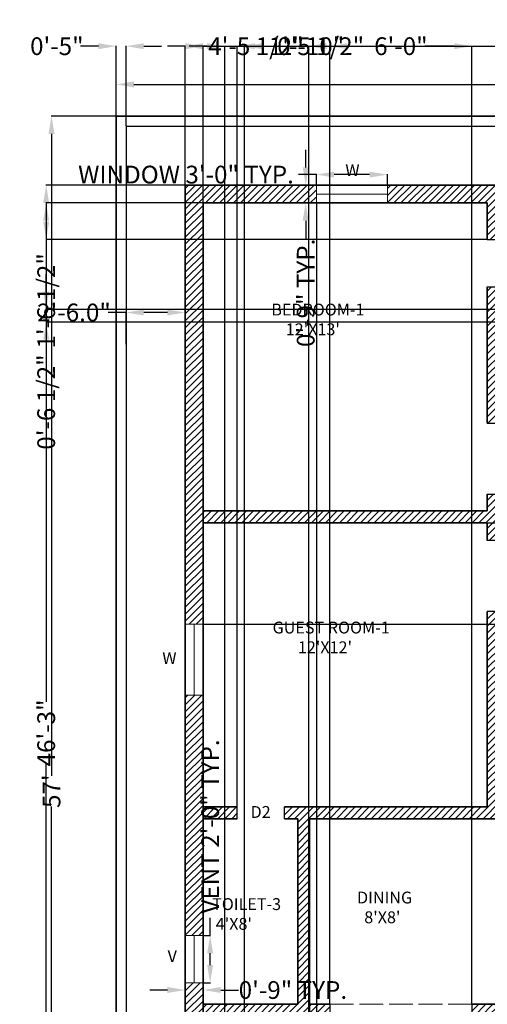
# Model space of a CAD drawing. Units: inches. Extents: x 287 to 864, y 208 to 990.
# Tile 2 of 3: x 287 to 524, y 491 to 990. Entities that reach past the tile are written whole.
import ezdxf

# ---------------------------------------------------------------- set-up
doc = ezdxf.new("R2010")
doc.units = ezdxf.units.IN
doc.header["$MEASUREMENT"] = 0
doc.linetypes.add('ACAD_ISO02W100', pattern=[15, 12, -3])
for name, color, linetype, lineweight in [('A-ANNO-DIMS', 2, 'Continuous', 18), ('A-ANNO-TEXT', 7, 'Continuous', 18), ('A-AREA-IDEN', 7, 'Continuous', 18), ('A-DOOR', 3, 'Continuous', 25), ('A-GLAZ', 4, 'Continuous', 18), ('A-SITE-WALL', 7, 'Continuous', 30), ('A-WALL', 7, 'Continuous', 35), ('A-WALL-OVHD', 7, 'ACAD_ISO02W100', 18), ('C-PROP', 7, 'Continuous', 35)]:
    doc.layers.add(name, color=color, linetype=linetype, lineweight=lineweight)
doc.layers.add('A-WALL-PATT', color=240, linetype='Continuous', lineweight=13, true_color=0xed1f24)
doc.styles.get("Standard").update_dxf_attribs({"font": 'arial.ttf'})
doc.dimstyles.get("Standard").update_dxf_attribs({"dimtxt": 9, "dimasz": 9, "dimexe": 0.18, "dimexo": 0.0625, "dimgap": 0.09, "dimtad": 0, "dimdec": 1, "dimzin": 0, "dimdsep": 46, "dimlunit": 3, "dimtxsty": 'Standard', "dimcen": 0.09, "dimadec": 0, "dimazin": 0, "dimtfac": 1, "dimtdec": 1, "dimtofl": 0, "dimtmove": 0, "dimatfit": 3, "dimfxl": 1, "dimtolj": 1, "dimtzin": 0, "dimarcsym": 0})

# ---------------------------------------------------------------- blocks, each defined once
blk = doc.blocks.new('*D1')
at = {"layer": 'A-ANNO-DIMS', "color": 0, "lineweight": -2, "transparency": 16777216}
for p, q in [((335.59, 941.12), (335.59, 957.32)), ((344.59, 957.14), (567.68, 957.14)), ((806.59, 957.14), (583.5, 957.14)), ((815.59, 941.12), (815.59, 957.32))]:
    blk.add_line(p, q, dxfattribs=at)
at = {"layer": 'A-ANNO-DIMS', "color": 0, "transparency": 16777216}
for points in [[(344.59, 958.64), (344.59, 955.64), (335.59, 957.14)], [(806.59, 958.64), (806.59, 955.64), (815.59, 957.14)]]:
    blk.add_solid(points, dxfattribs=at)
at = {"layer": 'Defpoints', "color": 0, "transparency": 16777216}
for p in [(815.59, 957.14), (335.59, 941.05), (815.59, 941.05)]:
    blk.add_point(p, dxfattribs=at)
at = {"layer": 'A-ANNO-DIMS', "color": 0, "transparency": 16777216, "insert": (575.59, 957.14), "char_height": 9, "attachment_point": 5}
blk.add_mtext("\\A1;40'", dxfattribs=at)
blk = doc.blocks.new('*D2')
at = {"layer": 'A-ANNO-DIMS', "color": 0, "lineweight": -2, "transparency": 16777216}
for p, q in [((335.53, 941.05), (302.65, 941.05)), ((302.83, 932.05), (302.83, 606.78)), ((302.83, 266.05), (302.83, 591.33)), ((335.53, 257.05), (302.65, 257.05))]:
    blk.add_line(p, q, dxfattribs=at)
at = {"layer": 'A-ANNO-DIMS', "color": 0, "transparency": 16777216}
for points in [[(301.33, 932.05), (304.33, 932.05), (302.83, 941.05)], [(301.33, 266.05), (304.33, 266.05), (302.83, 257.05)]]:
    blk.add_solid(points, dxfattribs=at)
at = {"layer": 'Defpoints', "color": 0, "transparency": 16777216}
for p in [(335.59, 941.05), (302.83, 257.05), (335.59, 257.05)]:
    blk.add_point(p, dxfattribs=at)
at = {"layer": 'A-ANNO-DIMS', "color": 0, "transparency": 16777216, "insert": (302.83, 599.05), "char_height": 9, "attachment_point": 5, "rotation": 90}
blk.add_mtext("\\A1;57'", dxfattribs=at)
blk = doc.blocks.new('*D3')
at = {"layer": 'A-ANNO-DIMS', "color": 0, "lineweight": -2, "transparency": 16777216}
for p, q in [((340.59, 841.58), (331.59, 841.58)), ((340.59, 825.53), (340.59, 841.76)), ((361.59, 841.58), (349.59, 841.58)), ((370.59, 825.53), (370.59, 841.76))]:
    blk.add_line(p, q, dxfattribs=at)
at = {"layer": 'A-ANNO-DIMS', "color": 0, "transparency": 16777216}
for points in [[(349.59, 843.08), (349.59, 840.08), (340.59, 841.58)], [(361.59, 843.08), (361.59, 840.08), (370.59, 841.58)]]:
    blk.add_solid(points, dxfattribs=at)
at = {"layer": 'Defpoints', "color": 0, "transparency": 16777216}
for p in [(340.59, 841.58), (340.59, 825.47), (370.59, 825.47)]:
    blk.add_point(p, dxfattribs=at)
at = {"layer": 'A-ANNO-DIMS', "color": 0, "transparency": 16777216, "insert": (314.22, 841.58), "char_height": 9, "attachment_point": 5}
blk.add_mtext('\\A1;2\'-6.0"', dxfattribs=at)
blk = doc.blocks.new('WIN-36IN')
for p, q in [((0, 9), (0, 0)), ((36, 9), (36, 0)), ((0, 4.5), (36, 4.5))]:
    blk.add_line(p, q)
blk = doc.blocks.new('VENT-24IN')
for p, q in [((0, 24), (9, 24)), ((4.5, 0), (4.5, 24)), ((0, 0), (9, 0))]:
    blk.add_line(p, q)
blk = doc.blocks.new('DOOR-OPENING-36IN')
for p, q in [((0, 36), (6, 36)), ((0, 0), (6, 0))]:
    blk.add_line(p, q)
blk = doc.blocks.new('DOOR-OPENING-24IN')
for p, q in [((0, 24), (6, 24)), ((0, 0), (6, 0))]:
    blk.add_line(p, q)
blk = doc.blocks.new('*D13')
at = {"layer": 'A-ANNO-DIMS', "color": 0, "lineweight": -2, "transparency": 16777216}
for p, q in [((436.99, 911.45), (427.99, 911.45)), ((436.99, 906.12), (436.99, 911.63)), ((463.99, 911.45), (445.99, 911.45)), ((472.99, 906.12), (472.99, 911.63))]:
    blk.add_line(p, q, dxfattribs=at)
at = {"layer": 'A-ANNO-DIMS', "color": 0, "transparency": 16777216}
for points in [[(445.99, 912.95), (445.99, 909.95), (436.99, 911.45)], [(463.99, 912.95), (463.99, 909.95), (472.99, 911.45)]]:
    blk.add_solid(points, dxfattribs=at)
at = {"layer": 'Defpoints', "color": 0, "transparency": 16777216}
for p in [(436.99, 911.45), (436.99, 906.05), (472.99, 906.05)]:
    blk.add_point(p, dxfattribs=at)
at = {"layer": 'A-ANNO-DIMS', "color": 0, "transparency": 16777216, "insert": (370.96, 911.45), "char_height": 9, "attachment_point": 5}
blk.add_mtext('\\A1;WINDOW 3\'-0" TYP.', dxfattribs=at)
blk = doc.blocks.new('*D14')
at = {"layer": 'A-ANNO-DIMS', "color": 0, "lineweight": -2, "transparency": 16777216}
for p, q in [((431.59, 915.05), (431.59, 924.05)), ((436.93, 906.05), (431.41, 906.05)), ((436.93, 897.05), (431.41, 897.05)), ((431.59, 888.05), (431.59, 879.05))]:
    blk.add_line(p, q, dxfattribs=at)
at = {"layer": 'A-ANNO-DIMS', "color": 0, "transparency": 16777216}
for points in [[(430.09, 915.05), (433.09, 915.05), (431.59, 906.05)], [(430.09, 888.05), (433.09, 888.05), (431.59, 897.05)]]:
    blk.add_solid(points, dxfattribs=at)
at = {"layer": 'Defpoints', "color": 0, "transparency": 16777216}
for p in [(436.99, 906.05), (431.59, 897.05), (436.99, 897.05)]:
    blk.add_point(p, dxfattribs=at)
at = {"layer": 'A-ANNO-DIMS', "color": 0, "transparency": 16777216, "insert": (431.59, 851.53), "char_height": 9, "attachment_point": 5, "rotation": 90}
blk.add_mtext('\\A1;0\'-9" TYP.', dxfattribs=at)
blk = doc.blocks.new('*D19')
at = {"layer": 'A-ANNO-DIMS', "color": 0, "lineweight": -2, "transparency": 16777216}
for p, q in [((383.19, 525.9), (383.19, 534.9)), ((379.65, 525.9), (383.37, 525.9)), ((383.19, 510.9), (383.19, 516.9)), ((379.65, 501.9), (383.37, 501.9))]:
    blk.add_line(p, q, dxfattribs=at)
at = {"layer": 'A-ANNO-DIMS', "color": 0, "transparency": 16777216}
for points in [[(381.69, 516.9), (384.69, 516.9), (383.19, 525.9)], [(381.69, 510.9), (384.69, 510.9), (383.19, 501.9)]]:
    blk.add_solid(points, dxfattribs=at)
at = {"layer": 'Defpoints', "color": 0, "transparency": 16777216}
for p in [(379.59, 525.9), (383.19, 525.9), (379.59, 501.9)]:
    blk.add_point(p, dxfattribs=at)
at = {"layer": 'A-ANNO-DIMS', "color": 0, "transparency": 16777216, "insert": (383.19, 581.17), "char_height": 9, "attachment_point": 5, "rotation": 90}
blk.add_mtext('\\A1;VENT 2\'-0" TYP.', dxfattribs=at)
blk = doc.blocks.new('*D20')
at = {"layer": 'A-ANNO-DIMS', "color": 0, "lineweight": -2, "transparency": 16777216}
for p, q in [((370.59, 501.84), (370.59, 498.12)), ((379.59, 501.84), (379.59, 498.12)), ((361.59, 498.3), (352.59, 498.3)), ((388.59, 498.3), (397.59, 498.3))]:
    blk.add_line(p, q, dxfattribs=at)
at = {"layer": 'A-ANNO-DIMS', "color": 0, "transparency": 16777216}
for points in [[(361.59, 499.8), (361.59, 496.8), (370.59, 498.3)], [(388.59, 499.8), (388.59, 496.8), (379.59, 498.3)]]:
    blk.add_solid(points, dxfattribs=at)
at = {"layer": 'Defpoints', "color": 0, "transparency": 16777216}
for p in [(370.59, 501.9), (379.59, 501.9), (379.59, 498.3)]:
    blk.add_point(p, dxfattribs=at)
at = {"layer": 'A-ANNO-DIMS', "color": 0, "transparency": 16777216, "insert": (425.11, 498.3), "char_height": 9, "attachment_point": 5}
blk.add_mtext('\\A1;0\'-9" TYP.', dxfattribs=at)
blk = doc.blocks.new('*D23')
at = {"layer": 'A-ANNO-DIMS', "color": 0, "lineweight": -2, "transparency": 16777216}
for p, q in [((370.59, 906.12), (370.59, 976.68)), ((379.59, 976.5), (556.04, 976.5)), ((763.59, 976.5), (587.14, 976.5)), ((772.59, 906.12), (772.59, 976.68))]:
    blk.add_line(p, q, dxfattribs=at)
at = {"layer": 'A-ANNO-DIMS', "color": 0, "transparency": 16777216}
for points in [[(379.59, 978), (379.59, 975), (370.59, 976.5)], [(763.59, 978), (763.59, 975), (772.59, 976.5)]]:
    blk.add_solid(points, dxfattribs=at)
at = {"layer": 'Defpoints', "color": 0, "transparency": 16777216}
for p in [(772.59, 976.5), (370.59, 906.05), (772.59, 906.05)]:
    blk.add_point(p, dxfattribs=at)
at = {"layer": 'A-ANNO-DIMS', "color": 0, "transparency": 16777216, "insert": (571.59, 976.5), "char_height": 9, "attachment_point": 5}
blk.add_mtext('\\A1;33\'-6"', dxfattribs=at)
blk = doc.blocks.new('*D24')
at = {"layer": 'A-ANNO-DIMS', "color": 0, "lineweight": -2, "transparency": 16777216}
for p, q in [((370.53, 906.05), (299.96, 906.05)), ((300.14, 897.05), (300.14, 644.28)), ((300.14, 360.05), (300.14, 612.83)), ((370.53, 351.05), (299.96, 351.05))]:
    blk.add_line(p, q, dxfattribs=at)
at = {"layer": 'A-ANNO-DIMS', "color": 0, "transparency": 16777216}
for points in [[(298.64, 897.05), (301.64, 897.05), (300.14, 906.05)], [(298.64, 360.05), (301.64, 360.05), (300.14, 351.05)]]:
    blk.add_solid(points, dxfattribs=at)
at = {"layer": 'Defpoints', "color": 0, "transparency": 16777216}
for p in [(300.14, 906.05), (370.59, 906.05), (370.59, 351.05)]:
    blk.add_point(p, dxfattribs=at)
at = {"layer": 'A-ANNO-DIMS', "color": 0, "transparency": 16777216, "insert": (300.14, 628.55), "char_height": 9, "attachment_point": 5, "rotation": 90}
blk.add_mtext('\\A1;46\'-3"', dxfattribs=at)
blk = doc.blocks.new('*D28')
at = {"layer": 'A-ANNO-DIMS', "color": 0, "lineweight": -2, "transparency": 16777216}
for p, q in [((381.59, 976.5), (372.59, 976.5)), ((390.59, 351.12), (390.59, 976.68)), ((400.59, 351.12), (400.59, 976.68)), ((409.59, 976.5), (418.59, 976.5))]:
    blk.add_line(p, q, dxfattribs=at)
at = {"layer": 'A-ANNO-DIMS', "color": 0, "transparency": 16777216}
for points in [[(381.59, 978), (381.59, 975), (390.59, 976.5)], [(409.59, 978), (409.59, 975), (400.59, 976.5)]]:
    blk.add_solid(points, dxfattribs=at)
at = {"layer": 'Defpoints', "color": 0, "transparency": 16777216}
for p in [(400.59, 976.5), (390.59, 351.05), (400.59, 351.05)]:
    blk.add_point(p, dxfattribs=at)
at = {"layer": 'A-ANNO-DIMS', "color": 0, "transparency": 16777216, "insert": (434.14, 976.5), "char_height": 9, "attachment_point": 5}
blk.add_mtext('\\A1;0\'-10"', dxfattribs=at)
blk = doc.blocks.new('*D31')
at = {"layer": 'A-ANNO-DIMS', "color": 0, "lineweight": -2, "transparency": 16777216}
for p, q in [((443.82, 491.12), (443.82, 976.68)), ((452.82, 976.5), (467.75, 976.5)), ((506.82, 976.5), (491.9, 976.5)), ((515.82, 491.12), (515.82, 976.68))]:
    blk.add_line(p, q, dxfattribs=at)
at = {"layer": 'A-ANNO-DIMS', "color": 0, "transparency": 16777216}
for points in [[(452.82, 978), (452.82, 975), (443.82, 976.5)], [(506.82, 978), (506.82, 975), (515.82, 976.5)]]:
    blk.add_solid(points, dxfattribs=at)
at = {"layer": 'Defpoints', "color": 0, "transparency": 16777216}
for p in [(515.82, 976.5), (443.82, 491.05), (515.82, 491.05)]:
    blk.add_point(p, dxfattribs=at)
at = {"layer": 'A-ANNO-DIMS', "color": 0, "transparency": 16777216, "insert": (479.82, 976.5), "char_height": 9, "attachment_point": 5}
blk.add_mtext('\\A1;6\'-0"', dxfattribs=at)
blk = doc.blocks.new('*D32')
at = {"layer": 'A-ANNO-DIMS', "color": 0, "lineweight": -2, "transparency": 16777216}
for p, q in [((433.59, 490.99), (433.59, 221.42)), ((443.82, 484.99), (443.82, 221.42)), ((424.59, 221.6), (415.59, 221.6)), ((452.82, 221.6), (461.82, 221.6))]:
    blk.add_line(p, q, dxfattribs=at)
at = {"layer": 'A-ANNO-DIMS', "color": 0, "transparency": 16777216}
for points in [[(424.59, 223.1), (424.59, 220.1), (433.59, 221.6)], [(452.82, 223.1), (452.82, 220.1), (443.82, 221.6)]]:
    blk.add_solid(points, dxfattribs=at)
at = {"layer": 'Defpoints', "color": 0, "transparency": 16777216}
for p in [(433.59, 491.05), (443.82, 485.05), (443.82, 221.6)]:
    blk.add_point(p, dxfattribs=at)
at = {"layer": 'A-ANNO-DIMS', "color": 0, "transparency": 16777216, "insert": (477.37, 221.6), "char_height": 9, "attachment_point": 5}
blk.add_mtext('\\A1;0\'-10"', dxfattribs=at)
blk = doc.blocks.new('*D33')
at = {"layer": 'A-ANNO-DIMS', "color": 0, "lineweight": -2, "transparency": 16777216}
for p, q in [((379.59, 896.99), (379.59, 221.42)), ((436.99, 896.99), (436.99, 221.42)), ((370.59, 221.6), (361.59, 221.6)), ((445.99, 221.6), (454.99, 221.6))]:
    blk.add_line(p, q, dxfattribs=at)
at = {"layer": 'A-ANNO-DIMS', "color": 0, "transparency": 16777216}
for points in [[(370.59, 223.1), (370.59, 220.1), (379.59, 221.6)], [(445.99, 223.1), (445.99, 220.1), (436.99, 221.6)]]:
    blk.add_solid(points, dxfattribs=at)
at = {"layer": 'Defpoints', "color": 0, "transparency": 16777216}
for p in [(379.59, 897.05), (436.99, 897.05), (436.99, 221.6)]:
    blk.add_point(p, dxfattribs=at)
at = {"layer": 'A-ANNO-DIMS', "color": 0, "transparency": 16777216, "insert": (408.29, 221.6), "char_height": 9, "attachment_point": 5}
blk.add_mtext('\\A1;4\'-9 1/2"', dxfattribs=at)
blk = doc.blocks.new('*D36')
at = {"layer": 'A-ANNO-DIMS', "color": 0, "lineweight": -2, "transparency": 16777216}
for p, q in [((851.039945, 744.054509), (851.039945, 753.054509)), ((379.652445, 735.054509), (851.219945, 735.054509)), ((379.652445, 683.646477), (851.219945, 683.646477)), ((851.039945, 674.646477), (851.039945, 665.646477))]:
    blk.add_line(p, q, dxfattribs=at)
at = {"layer": 'A-ANNO-DIMS', "color": 0, "transparency": 16777216}
for points in [[(849.539945, 744.054509), (852.539945, 744.054509), (851.039945, 735.054509)], [(849.539945, 674.646477), (852.539945, 674.646477), (851.039945, 683.646477)]]:
    blk.add_solid(points, dxfattribs=at)
at = {"layer": 'Defpoints', "color": 0, "transparency": 16777216}
for p in [(379.589945, 735.054509), (379.589945, 683.646477), (851.039945, 683.646477)]:
    blk.add_point(p, dxfattribs=at)
at = {"layer": 'A-ANNO-DIMS', "color": 0, "transparency": 16777216, "insert": (851.039945, 709.350493), "char_height": 9, "attachment_point": 5, "rotation": 90}
blk.add_mtext('\\A1;4\'-3 1/2"', dxfattribs=at)
blk = doc.blocks.new('*D39')
at = {"layer": 'A-ANNO-DIMS', "color": 0, "lineweight": -2, "transparency": 16777216}
for p, q in [((370.59, 976.5), (361.59, 976.5)), ((379.59, 360.12), (379.59, 976.68)), ((433.14, 360.12), (433.14, 976.68)), ((442.14, 976.5), (451.14, 976.5))]:
    blk.add_line(p, q, dxfattribs=at)
at = {"layer": 'A-ANNO-DIMS', "color": 0, "transparency": 16777216}
for points in [[(370.59, 978), (370.59, 975), (379.59, 976.5)], [(442.14, 978), (442.14, 975), (433.14, 976.5)]]:
    blk.add_solid(points, dxfattribs=at)
at = {"layer": 'Defpoints', "color": 0, "transparency": 16777216}
for p in [(433.14, 976.5), (379.59, 360.05), (433.14, 360.05)]:
    blk.add_point(p, dxfattribs=at)
at = {"layer": 'A-ANNO-DIMS', "color": 0, "transparency": 16777216, "insert": (406.37, 976.5), "char_height": 9, "attachment_point": 5}
blk.add_mtext('\\A1;4\'-5 1/2"', dxfattribs=at)
blk = doc.blocks.new('*D42')
at = {"layer": 'A-ANNO-DIMS', "color": 0, "lineweight": -2, "transparency": 16777216}
for p, q in [((523.53, 897.05), (299.96, 897.05)), ((300.14, 888.05), (300.14, 887.59)), ((523.53, 878.59), (299.96, 878.59)), ((300.14, 878.59), (300.14, 869.59))]:
    blk.add_line(p, q, dxfattribs=at)
at = {"layer": 'A-ANNO-DIMS', "color": 0, "transparency": 16777216}
for points in [[(298.64, 888.05), (301.64, 888.05), (300.14, 897.05)], [(298.64, 887.59), (301.64, 887.59), (300.14, 878.59)]]:
    blk.add_solid(points, dxfattribs=at)
at = {"layer": 'Defpoints', "color": 0, "transparency": 16777216}
for p in [(523.59, 897.05), (300.14, 878.59), (523.59, 878.59)]:
    blk.add_point(p, dxfattribs=at)
at = {"layer": 'A-ANNO-DIMS', "color": 0, "transparency": 16777216, "insert": (300.14, 847.47), "char_height": 9, "attachment_point": 5, "rotation": 90}
blk.add_mtext('\\A1;1\'-6 1/2"', dxfattribs=at)
blk = doc.blocks.new('*D43')
at = {"layer": 'A-ANNO-DIMS', "color": 0, "lineweight": -2, "transparency": 16777216}
for p, q in [((300.14, 852.05), (300.14, 861.05)), ((613.53, 843.05), (299.96, 843.05)), ((613.53, 836.74), (299.96, 836.74)), ((300.14, 827.74), (300.14, 818.74))]:
    blk.add_line(p, q, dxfattribs=at)
at = {"layer": 'A-ANNO-DIMS', "color": 0, "transparency": 16777216}
for points in [[(298.64, 852.05), (301.64, 852.05), (300.14, 843.05)], [(298.64, 827.74), (301.64, 827.74), (300.14, 836.74)]]:
    blk.add_solid(points, dxfattribs=at)
at = {"layer": 'Defpoints', "color": 0, "transparency": 16777216}
for p in [(613.59, 843.05), (300.14, 836.74), (613.59, 836.74)]:
    blk.add_point(p, dxfattribs=at)
at = {"layer": 'A-ANNO-DIMS', "color": 0, "transparency": 16777216, "insert": (300.14, 796.2), "char_height": 9, "attachment_point": 5, "rotation": 90}
blk.add_mtext('\\A1;0\'-6 1/2"', dxfattribs=at)
blk = doc.blocks.new('*D46')
at = {"layer": 'A-ANNO-DIMS', "color": 0, "lineweight": -2, "transparency": 16777216}
for p, q in [((370.59, 976.5), (361.59, 976.5)), ((379.59, 591.12), (379.59, 976.68)), ((396.92, 591.12), (396.92, 976.68)), ((405.92, 976.5), (414.92, 976.5))]:
    blk.add_line(p, q, dxfattribs=at)
at = {"layer": 'A-ANNO-DIMS', "color": 0, "transparency": 16777216}
for points in [[(370.59, 978), (370.59, 975), (379.59, 976.5)], [(405.92, 978), (405.92, 975), (396.92, 976.5)]]:
    blk.add_solid(points, dxfattribs=at)
at = {"layer": 'Defpoints', "color": 0, "transparency": 16777216}
for p in [(396.92, 976.5), (379.59, 591.05), (396.92, 591.05)]:
    blk.add_point(p, dxfattribs=at)
at = {"layer": 'A-ANNO-DIMS', "color": 0, "transparency": 16777216, "insert": (437.04, 976.5), "char_height": 9, "attachment_point": 5}
blk.add_mtext('\\A1;1\'-5 1/2"', dxfattribs=at)
blk = doc.blocks.new('*D51')
at = {"layer": 'A-ANNO-DIMS', "color": 0, "lineweight": -2, "transparency": 16777216}
for p, q in [((326.59, 976.5), (317.59, 976.5)), ((335.59, 941.12), (335.59, 976.68)), ((340.59, 936.12), (340.59, 976.68)), ((349.59, 976.5), (358.59, 976.5))]:
    blk.add_line(p, q, dxfattribs=at)
at = {"layer": 'A-ANNO-DIMS', "color": 0, "transparency": 16777216}
for points in [[(326.59, 978), (326.59, 975), (335.59, 976.5)], [(349.59, 978), (349.59, 975), (340.59, 976.5)]]:
    blk.add_solid(points, dxfattribs=at)
at = {"layer": 'Defpoints', "color": 0, "transparency": 16777216}
for p in [(335.59, 976.5), (335.59, 941.05), (340.59, 936.05)]:
    blk.add_point(p, dxfattribs=at)
at = {"layer": 'A-ANNO-DIMS', "color": 0, "transparency": 16777216, "insert": (305.54, 976.5), "char_height": 9, "attachment_point": 5}
blk.add_mtext('\\A1;0\'-5"', dxfattribs=at)

msp = doc.modelspace()

# ---------------------------------------------------------------- hatches: boundary and pattern name
at = {"layer": 'A-WALL-PATT'}
h = msp.add_hatch(dxfattribs=at)
h.set_pattern_fill('ANSI31', color=256, scale=20)
h.paths.add_polyline_path([(443.82, 491.05), (433.59, 491.05), (433.59, 585.05), (529.59, 585.05), (529.59, 690.13), (523.59, 690.13), (523.59, 591.05), (420.92, 591.05), (420.92, 585.05), (427.59, 585.05), (427.59, 491.05), (379.59, 491.05), (379.59, 501.9), (370.59, 501.9), (370.59, 351.05), (433.14, 351.05), (433.14, 360.05), (379.59, 360.05), (379.59, 485.05), (443.82, 485.05)])
h.paths.add_polyline_path([(616.36, 360.05), (469.14, 360.05), (469.14, 351.05), (616.36, 351.05)])
h.paths.add_polyline_path([(772.59, 647.65), (763.59, 647.65), (763.59, 591.05), (753.41, 591.05), (753.41, 585.05), (763.59, 585.05), (763.59, 525.9), (772.59, 525.9)])
h.paths.add_polyline_path([(772.59, 906.05), (714.78, 906.05), (714.78, 897.05), (763.59, 897.05), (763.59, 741.05), (619.59, 741.05), (619.59, 749.52), (613.59, 749.52), (613.59, 637.13), (619.59, 637.13), (619.59, 735.05), (763.59, 735.05), (763.59, 683.65), (772.59, 683.65)])
h.paths.add_polyline_path([(678.78, 906.05), (581.92, 906.05), (581.92, 897.05), (613.59, 897.05), (613.59, 849.05), (529.59, 849.05), (529.59, 854.59), (523.59, 854.59), (523.59, 785.52), (529.59, 785.52), (529.59, 789.05), (613.59, 789.05), (613.59, 785.52), (619.59, 785.52), (619.59, 812.74), (613.59, 812.74), (613.59, 795.05), (529.59, 795.05), (529.59, 843.05), (613.59, 843.05), (613.59, 836.74), (619.59, 836.74), (619.59, 897.05), (678.78, 897.05)])
h.paths.add_polyline_path([(557.92, 906.05), (472.99, 906.05), (472.99, 897.05), (523.59, 897.05), (523.59, 878.59), (529.59, 878.59), (529.59, 897.05), (557.92, 897.05)])
h.paths.add_polyline_path([(436.99, 906.05), (370.59, 906.05), (370.59, 683.65), (379.59, 683.65), (379.59, 735.05), (523.59, 735.05), (523.59, 726.13), (529.59, 726.13), (529.59, 749.52), (523.59, 749.52), (523.59, 741.05), (379.59, 741.05), (379.59, 897.05), (436.99, 897.05)])
h.paths.add_polyline_path([(379.59, 647.65), (370.59, 647.65), (370.59, 525.9), (379.59, 525.9), (379.59, 585.05), (396.92, 585.05), (396.92, 591.05), (379.59, 591.05)], flags=17)
h.paths.add_polyline_path([(529.59, 491.05), (515.82, 491.05), (515.82, 485.05), (523.59, 485.05), (523.59, 360.05), (529.59, 360.05)], flags=17)
h.paths.add_polyline_path([(763.59, 444.61), (772.59, 444.61), (772.59, 501.9), (763.59, 501.9), (763.59, 491.05), (703.59, 491.05), (703.59, 585.05), (729.41, 585.05), (729.41, 591.05), (619.59, 591.05), (619.59, 601.13), (613.59, 601.13), (613.59, 585.05), (697.59, 585.05), (697.59, 485.05), (763.59, 485.05)])
h.paths.add_polyline_path([(772.59, 408.61), (763.59, 408.61), (763.59, 360.05), (712.36, 360.05), (712.36, 351.05), (772.59, 351.05)])

# ---------------------------------------------------------------- linework, layer by layer
at = {"layer": 'A-DOOR'}
for p, q in [((443.82, 491.05), (443.82, 485.05)), ((515.82, 491.05), (515.82, 485.05))]:
    msp.add_line(p, q, dxfattribs=at)
at = {"layer": 'A-SITE-WALL'}
for q in [(810.59, 936.05), (340.59, 266.05)]:
    msp.add_line((340.59, 936.05), q, dxfattribs=at)
at = {"layer": 'A-WALL'}
for p, q in [((370.59, 351.05), (370.59, 906.05)), ((370.59, 906.05), (772.59, 906.05)), ((379.59, 897.05), (523.59, 897.05)), ((379.59, 741.05), (379.59, 897.05)), ((523.59, 878.59), (523.59, 897.05)), ((523.59, 785.52), (523.59, 854.59)), ((523.59, 741.05), (523.59, 749.52)), ((379.59, 741.05), (523.59, 741.05)), ((379.59, 735.05), (523.59, 735.05)), ((379.59, 591.05), (379.59, 735.05)), ((523.59, 726.13), (523.59, 735.05)), ((523.59, 591.05), (523.59, 690.13)), ((379.59, 591.05), (396.92, 591.05)), ((420.92, 591.05), (523.59, 591.05)), ((379.59, 585.05), (396.92, 585.05)), ((379.59, 491.05), (379.59, 585.05)), ((420.92, 585.05), (427.59, 585.05)), ((427.59, 491.05), (427.59, 585.05)), ((433.59, 491.05), (433.59, 585.05)), ((433.59, 585.05), (529.59, 585.05)), ((427.59, 491.05), (379.59, 491.05)), ((443.82, 491.05), (433.59, 491.05)), ((529.59, 491.05), (515.82, 491.05))]:
    msp.add_line(p, q, dxfattribs=at)
at = {"layer": 'A-WALL-OVHD'}
msp.add_line((443.82, 491.05), (515.82, 491.05), dxfattribs=at)
at = {"layer": 'C-PROP'}
for p, q in [((335.59, 941.05), (815.59, 941.05)), ((335.59, 257.05), (335.59, 941.05))]:
    msp.add_line(p, q, dxfattribs=at)

# ---------------------------------------------------------------- block references
at = {"layer": 'A-DOOR'}
for name, p in [('DOOR-OPENING-24IN', (523.59, 854.59)), ('DOOR-OPENING-36IN', (523.59, 749.52))]:
    msp.add_blockref(name, p, dxfattribs=at)
for name, p, rotation in [('DOOR-OPENING-36IN', (529.59, 726.13), 180), ('DOOR-OPENING-24IN', (420.92, 585.05), 89.9999999999993)]:
    msp.add_blockref(name, p, dxfattribs=dict(at, rotation=rotation))
at = {"layer": 'A-GLAZ'}
for p, rotation in [((472.99, 906.05), 180), ((370.59, 683.65), 269.9999999999999)]:
    msp.add_blockref('WIN-36IN', p, dxfattribs=dict(at, rotation=rotation))
msp.add_blockref('VENT-24IN', (370.59, 501.9), dxfattribs=at)

# ---------------------------------------------------------------- texts
at = {"layer": 'A-ANNO-TEXT', "char_height": 6, "attachment_point": 1}
for s, insert in [('W', (451.69, 916.65)), ('W', (358.97, 669.46)), ('D2', (403.67, 591.51)), ('V', (361.65, 518.44))]:
    msp.add_mtext_dynamic_manual_height_columns(s, width=80.3005, gutter_width=1, heights=[0], dxfattribs=dict(at, insert=insert))
at = {"layer": 'A-AREA-IDEN', "char_height": 6, "attachment_point": 1}
for s, insert in [("BEDROOM-1\\P    12'X13'", (414.16, 846.05)), ("GUEST ROOM-1\\P       12'X12'", (414.82, 684.94)), ("TOILET-3\\P 4'X8'", (384.2, 544.82)), ("DINING\\P  8'X8'", (457.6, 548.15))]:
    msp.add_mtext_dynamic_manual_height_columns(s, width=80.3005, gutter_width=1, heights=[0], dxfattribs=dict(at, insert=insert))

# ---------------------------------------------------------------- dimensions: what is measured, and where the dimension line sits
at = {"layer": 'A-ANNO-DIMS'}
for base, p1, p2, override, picture, middle in [((433.1449, 976.5045), (379.5899, 360.0545), (433.1449, 360.0545), {"dimdec": 1, "dimlfac": 1, "dimrnd": 0, "dimzin": 1, "dimdsep": 46, "dimlunit": 4, "dimfrac": 2}, '*D39', (406.3674, 976.5045)), ((396.92, 976.5), (379.59, 591.05), (396.92, 591.05), {"dimdec": 1, "dimlfac": 1, "dimrnd": 0, "dimzin": 1, "dimdsep": 46, "dimlunit": 4, "dimfrac": 2}, '*D46', (437.04, 976.5)), ((335.59, 976.5), (340.59, 936.05), (335.59, 941.05), {"dimdec": 1, "dimlfac": 1, "dimrnd": 0, "dimzin": 1, "dimdsep": 46, "dimlunit": 4, "dimfrac": 2}, '*D51', (305.54, 976.5)), ((772.59, 976.5), (370.59, 906.05), (772.59, 906.05), {"dimdec": 1, "dimlfac": 1, "dimrnd": 0, "dimzin": 1, "dimdsep": 46, "dimlunit": 4, "dimfrac": 2}, '*D23', (571.59, 976.5)), ((400.59, 976.5), (390.59, 351.05), (400.59, 351.05), {"dimdec": 1, "dimlfac": 1, "dimrnd": 0, "dimzin": 1, "dimdsep": 46, "dimlunit": 4, "dimfrac": 2}, '*D28', (434.14, 976.5)), ((515.82, 976.5), (443.82, 491.05), (515.82, 491.05), {"dimdec": 1, "dimlfac": 1, "dimrnd": 0, "dimzin": 1, "dimdsep": 46, "dimlunit": 4, "dimfrac": 2}, '*D31', (479.82, 976.5)), ((815.59, 957.14), (335.59, 941.05), (815.59, 941.05), {"dimclrd": 0, "dimclre": 0, "dimclrt": 0}, '*D1', (575.59, 957.14)), ((436.99, 221.6), (379.59, 897.05), (436.99, 897.05), {"dimdec": 1, "dimlfac": 1, "dimrnd": 0, "dimzin": 1, "dimdsep": 46, "dimlunit": 4, "dimfrac": 2}, '*D33', (408.29, 221.6)), ((340.59, 841.58), (370.59, 825.47), (340.59, 825.47), {"dimclrd": 0, "dimclre": 0, "dimclrt": 0}, '*D3', (314.22, 841.58)), ((443.82, 221.6), (433.59, 491.05), (443.82, 485.05), {"dimdec": 1, "dimlfac": 1, "dimrnd": 0, "dimzin": 1, "dimdsep": 46, "dimlunit": 4, "dimfrac": 2}, '*D32', (477.37, 221.6))]:
    dim = msp.add_linear_dim(base=base, p1=p1, p2=p2, dimstyle='Standard', override=override, dxfattribs=at)
    dim.commit()
    dim.dimension.update_dxf_attribs({"geometry": picture, "text_midpoint": middle})
for base, p1, p2, override, picture, middle in [((302.83, 257.05), (335.59, 941.05), (335.59, 257.05), {"dimclrd": 0, "dimclre": 0, "dimclrt": 0}, '*D2', (302.83, 599.05)), ((300.14, 906.05), (370.59, 351.05), (370.59, 906.05), {"dimdec": 1, "dimlfac": 1, "dimrnd": 0, "dimzin": 1, "dimdsep": 46, "dimlunit": 4, "dimfrac": 2}, '*D24', (300.14, 628.55)), ((300.14, 878.59), (523.59, 897.05), (523.59, 878.59), {"dimdec": 1, "dimlfac": 1, "dimrnd": 0, "dimzin": 1, "dimdsep": 46, "dimlunit": 4, "dimfrac": 2}, '*D42', (300.14, 847.47)), ((300.14, 836.74), (613.59, 843.05), (613.59, 836.74), {"dimdec": 1, "dimlfac": 1, "dimrnd": 0, "dimzin": 1, "dimdsep": 46, "dimlunit": 4, "dimfrac": 2}, '*D43', (300.14, 796.2)), ((851.04, 683.65), (379.59, 735.05), (379.59, 683.65), {"dimdec": 1, "dimlfac": 1, "dimrnd": 0, "dimzin": 1, "dimdsep": 46, "dimlunit": 4, "dimfrac": 2}, '*D36', (851.04, 709.35))]:
    dim = msp.add_linear_dim(base=base, p1=p1, p2=p2, angle=90, dimstyle='Standard', override=override, dxfattribs=at)
    dim.commit()
    dim.dimension.update_dxf_attribs({"geometry": picture, "text_midpoint": middle})
for base, p1, p2, angle, text, picture, middle in [((436.99, 911.45), (472.99, 906.05), (436.99, 906.05), 180, 'WINDOW <> TYP.', '*D13', (370.96, 911.45)), ((431.59, 897.05), (436.99, 906.05), (436.99, 897.05), 270, '<> TYP.', '*D14', (431.59, 851.53)), ((383.19, 525.9), (379.59, 501.9), (379.59, 525.9), 90, 'VENT <> TYP.', '*D19', (383.19, 581.17))]:
    dim = msp.add_linear_dim(base=base, p1=p1, p2=p2, angle=angle, text=text, dimstyle='Standard', override={"dimdec": 1, "dimlfac": 1, "dimrnd": 0, "dimzin": 1, "dimdsep": 46, "dimlunit": 4, "dimfrac": 2}, dxfattribs=at)
    dim.commit()
    dim.dimension.update_dxf_attribs({"geometry": picture, "text_midpoint": middle})
dim = msp.add_linear_dim(base=(379.59, 498.3), p1=(370.59, 501.9), p2=(379.59, 501.9), text='<> TYP.', dimstyle='Standard', override={"dimdec": 1, "dimlfac": 1, "dimrnd": 0, "dimzin": 1, "dimdsep": 46, "dimlunit": 4, "dimfrac": 2}, dxfattribs=at)
dim.commit()
dim.dimension.update_dxf_attribs({"geometry": '*D20', "text_midpoint": (425.11, 498.3)})

doc.saveas('drawing.dxf')
